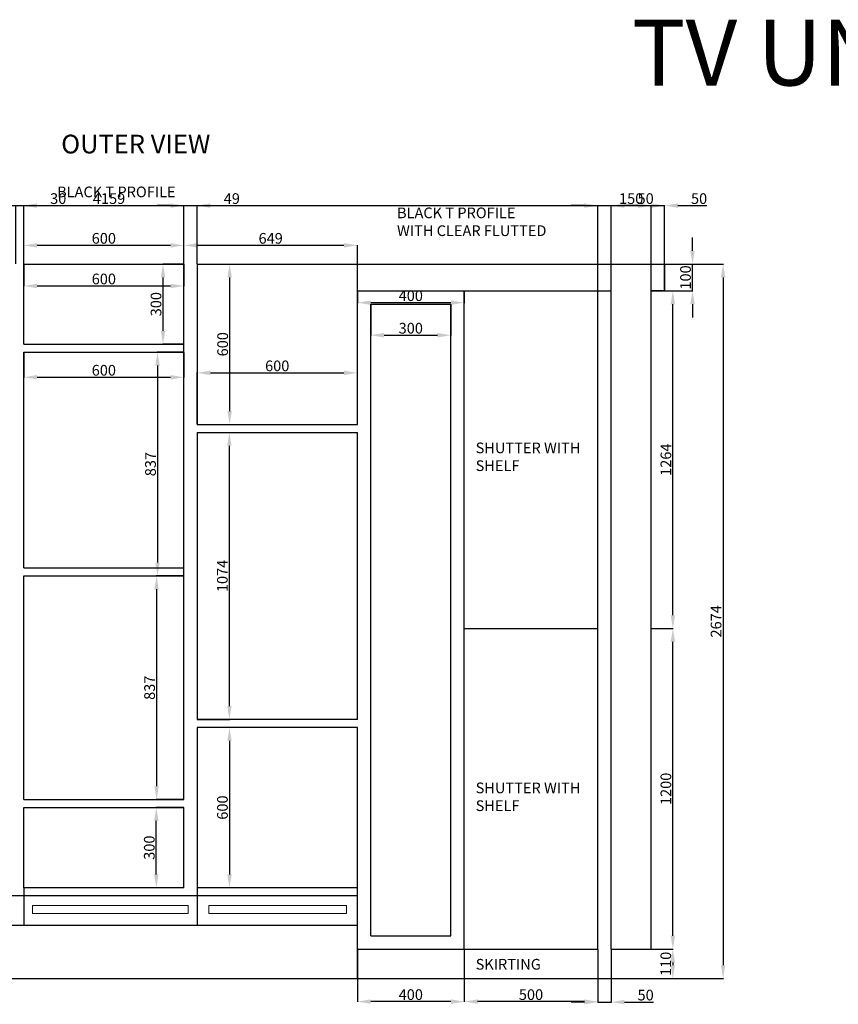
# Model space of a CAD drawing. Units: millimetres. Extents: x -2182 to 7969, y 257 to 4097.
# Tile 2 of 5: x -171 to 2894, y 412 to 4097. Entities that reach past the tile are written whole.
import ezdxf

# ---------------------------------------------------------------- set-up
doc = ezdxf.new("R2010")
doc.units = ezdxf.units.MM
for name, color, linetype, lineweight in [('A-ANNO-DIMS', 2, 'Continuous', 18), ('A-ANNO-TEXT', 3, 'Continuous', 18), ('A-ELEV', 7, 'Continuous', 25), ('A-FURN-HRDW', 8, 'Continuous', 18)]:
    doc.layers.add(name, color=color, linetype=linetype, lineweight=lineweight)
doc.styles.get("Standard").update_dxf_attribs({"font": 'arial.ttf'})
doc.dimstyles.new('ISO-25', dxfattribs={"dimtxt": 40, "dimasz": 50, "dimexe": 1.25, "dimexo": 0.625, "dimtad": 1, "dimtxsty": 'Standard', "dimcen": 2.5, "dimadec": 0, "dimazin": 0, "dimtfac": 1, "dimtmove": 0, "dimatfit": 3, "dimfxl": 1, "dimarcsym": 0})

# ---------------------------------------------------------------- blocks, each defined once
blk = doc.blocks.new('*D5')
at = {"layer": 'A-ANNO-DIMS', "color": 0, "lineweight": -2, "transparency": 16777216}
for p, q in [((2193.8, 618.5), (2275.3, 618.5)), ((2274.1, 568.5), (2274.1, 558.5)), ((2193.8, 508.5), (2275.3, 508.5))]:
    blk.add_line(p, q, dxfattribs=at)
at = {"layer": 'A-ANNO-DIMS', "color": 0, "transparency": 16777216}
for points in [[(2265.7, 568.5), (2282.4, 568.5), (2274.1, 618.5)], [(2265.7, 558.5), (2282.4, 558.5), (2274.1, 508.5)]]:
    blk.add_solid(points, dxfattribs=at)
at = {"layer": 'Defpoints', "color": 0, "transparency": 16777216}
for p in [(2193.2, 618.5), (2193.2, 508.5), (2274.1, 508.5)]:
    blk.add_point(p, dxfattribs=at)
at = {"layer": 'A-ANNO-DIMS', "color": 0, "transparency": 16777216, "insert": (2253, 563.5), "char_height": 40, "attachment_point": 5, "rotation": 90}
blk.add_mtext('110', dxfattribs=at)
blk = doc.blocks.new('*D6')
at = {"layer": 'A-ANNO-DIMS', "color": 0, "lineweight": -2, "transparency": 16777216}
for p, q in [((2193.8, 1818.5), (2275.6, 1818.5)), ((2274.3, 668.5), (2274.3, 1768.5)), ((2043.8, 618.5), (2275.6, 618.5))]:
    blk.add_line(p, q, dxfattribs=at)
at = {"layer": 'A-ANNO-DIMS', "color": 0, "transparency": 16777216}
for points in [[(2266, 1768.5), (2282.6, 1768.5), (2274.3, 1818.5)], [(2266, 668.5), (2282.6, 668.5), (2274.3, 618.5)]]:
    blk.add_solid(points, dxfattribs=at)
at = {"layer": 'Defpoints', "color": 0, "transparency": 16777216}
for p in [(2193.2, 1818.5), (2274.3, 1818.5), (2043.2, 618.5)]:
    blk.add_point(p, dxfattribs=at)
at = {"layer": 'A-ANNO-DIMS', "color": 0, "transparency": 16777216, "insert": (2253.3, 1218.5), "char_height": 40, "attachment_point": 5, "rotation": 90}
blk.add_mtext('1200', dxfattribs=at)
blk = doc.blocks.new('*D7')
at = {"layer": 'A-ANNO-DIMS', "color": 0, "lineweight": -2, "transparency": 16777216}
for p, q in [((2193.8, 3082.5), (2275.6, 3082.5)), ((2274.3, 1868.5), (2274.3, 3032.5)), ((2193.8, 1818.5), (2275.6, 1818.5))]:
    blk.add_line(p, q, dxfattribs=at)
at = {"layer": 'A-ANNO-DIMS', "color": 0, "transparency": 16777216}
for points in [[(2266, 3032.5), (2282.6, 3032.5), (2274.3, 3082.5)], [(2266, 1868.5), (2282.6, 1868.5), (2274.3, 1818.5)]]:
    blk.add_solid(points, dxfattribs=at)
at = {"layer": 'Defpoints', "color": 0, "transparency": 16777216}
for p in [(2193.2, 3082.5), (2274.3, 3082.5), (2193.2, 1818.5)]:
    blk.add_point(p, dxfattribs=at)
at = {"layer": 'A-ANNO-DIMS', "color": 0, "transparency": 16777216, "insert": (2253.3, 2450.5), "char_height": 40, "attachment_point": 5, "rotation": 90}
blk.add_mtext('1264', dxfattribs=at)
blk = doc.blocks.new('*D8')
at = {"layer": 'A-ANNO-DIMS', "color": 0, "lineweight": -2, "transparency": 16777216}
for p, q in [((2347.9, 3232.5), (2347.9, 3282.5)), ((2243.8, 3182.5), (2349.1, 3182.5)), ((2347.9, 3082.5), (2347.9, 3182.5)), ((2245.1, 3082.5), (2349.1, 3082.5)), ((2347.9, 3032.5), (2347.9, 2982.5))]:
    blk.add_line(p, q, dxfattribs=at)
at = {"layer": 'A-ANNO-DIMS', "color": 0, "transparency": 16777216}
for points in [[(2339.6, 3232.5), (2356.2, 3232.5), (2347.9, 3182.5)], [(2339.6, 3032.5), (2356.2, 3032.5), (2347.9, 3082.5)]]:
    blk.add_solid(points, dxfattribs=at)
at = {"layer": 'Defpoints', "color": 0, "transparency": 16777216}
for p in [(2243.2, 3182.5), (2347.9, 3182.5), (2244.4, 3082.5)]:
    blk.add_point(p, dxfattribs=at)
at = {"layer": 'A-ANNO-DIMS', "color": 0, "transparency": 16777216, "insert": (2326.8, 3132.5), "char_height": 40, "attachment_point": 5, "rotation": 90}
blk.add_mtext('100', dxfattribs=at)
blk = doc.blocks.new('*D9')
at = {"layer": 'A-ANNO-DIMS', "color": 0, "lineweight": -2, "transparency": 16777216}
for p, q in [((1993.2, 617.8), (1993.2, 419.3)), ((2043.2, 617.8), (2043.2, 419.3)), ((1943.2, 420.5), (1893.2, 420.5)), ((1993.2, 420.5), (2043.2, 420.5)), ((2093.2, 420.5), (2201.6, 420.5))]:
    blk.add_line(p, q, dxfattribs=at)
at = {"layer": 'A-ANNO-DIMS', "color": 0, "transparency": 16777216}
for points in [[(1943.2, 428.9), (1943.2, 412.2), (1993.2, 420.5)], [(2093.2, 428.9), (2093.2, 412.2), (2043.2, 420.5)]]:
    blk.add_solid(points, dxfattribs=at)
at = {"layer": 'Defpoints', "color": 0, "transparency": 16777216}
for p in [(1993.2, 618.5), (2043.2, 618.5), (1993.2, 420.5)]:
    blk.add_point(p, dxfattribs=at)
at = {"layer": 'A-ANNO-DIMS', "color": 0, "transparency": 16777216, "insert": (2172.4, 441.6), "char_height": 40, "attachment_point": 5}
blk.add_mtext('50', dxfattribs=at)
blk = doc.blocks.new('*D10')
at = {"layer": 'A-ANNO-DIMS', "color": 0, "lineweight": -2, "transparency": 16777216}
for p, q in [((1493.2, 617.8), (1493.2, 421)), ((1993.2, 617.8), (1993.2, 421)), ((1943.2, 422.3), (1543.2, 422.3))]:
    blk.add_line(p, q, dxfattribs=at)
at = {"layer": 'A-ANNO-DIMS', "color": 0, "transparency": 16777216}
for points in [[(1543.2, 430.6), (1543.2, 413.9), (1493.2, 422.3)], [(1943.2, 430.6), (1943.2, 413.9), (1993.2, 422.3)]]:
    blk.add_solid(points, dxfattribs=at)
at = {"layer": 'Defpoints', "color": 0, "transparency": 16777216}
for p in [(1493.2, 618.5), (1993.2, 618.5), (1493.2, 422.3)]:
    blk.add_point(p, dxfattribs=at)
at = {"layer": 'A-ANNO-DIMS', "color": 0, "transparency": 16777216, "insert": (1743.2, 443.3), "char_height": 40, "attachment_point": 5}
blk.add_mtext('500', dxfattribs=at)
blk = doc.blocks.new('*D11')
at = {"layer": 'A-ANNO-DIMS', "color": 0, "lineweight": -2, "transparency": 16777216}
for p, q in [((1093.2, 617.8), (1093.2, 421)), ((1493.2, 617.8), (1493.2, 421)), ((1443.2, 422.3), (1143.2, 422.3))]:
    blk.add_line(p, q, dxfattribs=at)
at = {"layer": 'A-ANNO-DIMS', "color": 0, "transparency": 16777216}
for points in [[(1143.2, 430.6), (1143.2, 413.9), (1093.2, 422.3)], [(1443.2, 430.6), (1443.2, 413.9), (1493.2, 422.3)]]:
    blk.add_solid(points, dxfattribs=at)
at = {"layer": 'Defpoints', "color": 0, "transparency": 16777216}
for p in [(1093.2, 618.5), (1493.2, 618.5), (1093.2, 422.3)]:
    blk.add_point(p, dxfattribs=at)
at = {"layer": 'A-ANNO-DIMS', "color": 0, "transparency": 16777216, "insert": (1293.2, 443.3), "char_height": 40, "attachment_point": 5}
blk.add_mtext('400', dxfattribs=at)
blk = doc.blocks.new('*D12')
at = {"layer": 'A-ANNO-DIMS', "color": 0, "lineweight": -2, "transparency": 16777216}
for p, q in [((493.2, 2583.1), (493.2, 2776.7)), ((543.2, 2775.4), (1043.2, 2775.4)), ((1093.2, 2583.1), (1093.2, 2776.7))]:
    blk.add_line(p, q, dxfattribs=at)
at = {"layer": 'A-ANNO-DIMS', "color": 0, "transparency": 16777216}
for points in [[(543.2, 2783.8), (543.2, 2767.1), (493.2, 2775.4)], [(1043.2, 2783.8), (1043.2, 2767.1), (1093.2, 2775.4)]]:
    blk.add_solid(points, dxfattribs=at)
at = {"layer": 'Defpoints', "color": 0, "transparency": 16777216}
for p in [(1093.2, 2775.4), (493.2, 2582.5), (1093.2, 2582.5)]:
    blk.add_point(p, dxfattribs=at)
at = {"layer": 'A-ANNO-DIMS', "color": 0, "transparency": 16777216, "insert": (793.2, 2796.5), "char_height": 40, "attachment_point": 5}
blk.add_mtext('600', dxfattribs=at)
blk = doc.blocks.new('*D13')
at = {"layer": 'A-ANNO-DIMS', "color": 0, "lineweight": -2, "transparency": 16777216}
for p, q in [((493.8, 3182.5), (616.4, 3182.5)), ((615.1, 3132.5), (615.1, 2632.5)), ((493.8, 2582.5), (616.4, 2582.5))]:
    blk.add_line(p, q, dxfattribs=at)
at = {"layer": 'A-ANNO-DIMS', "color": 0, "transparency": 16777216}
for points in [[(606.8, 3132.5), (623.5, 3132.5), (615.1, 3182.5)], [(606.8, 2632.5), (623.5, 2632.5), (615.1, 2582.5)]]:
    blk.add_solid(points, dxfattribs=at)
at = {"layer": 'Defpoints', "color": 0, "transparency": 16777216}
for p in [(493.2, 3182.5), (493.2, 2582.5), (615.1, 2582.5)]:
    blk.add_point(p, dxfattribs=at)
at = {"layer": 'A-ANNO-DIMS', "color": 0, "transparency": 16777216, "insert": (594.1, 2882.5), "char_height": 40, "attachment_point": 5, "rotation": 90}
blk.add_mtext('600', dxfattribs=at)
blk = doc.blocks.new('*D14')
at = {"layer": 'A-ANNO-DIMS', "color": 0, "lineweight": -2, "transparency": 16777216}
for p, q in [((493.8, 2552.5), (615.3, 2552.5)), ((614.1, 1528.5), (614.1, 2502.5)), ((493.8, 1478.5), (615.3, 1478.5))]:
    blk.add_line(p, q, dxfattribs=at)
at = {"layer": 'A-ANNO-DIMS', "color": 0, "transparency": 16777216}
for points in [[(605.8, 2502.5), (622.4, 2502.5), (614.1, 2552.5)], [(605.8, 1528.5), (622.4, 1528.5), (614.1, 1478.5)]]:
    blk.add_solid(points, dxfattribs=at)
at = {"layer": 'Defpoints', "color": 0, "transparency": 16777216}
for p in [(493.2, 2552.5), (614.1, 2552.5), (493.2, 1478.5)]:
    blk.add_point(p, dxfattribs=at)
at = {"layer": 'A-ANNO-DIMS', "color": 0, "transparency": 16777216, "insert": (593, 2015.5), "char_height": 40, "attachment_point": 5, "rotation": 90}
blk.add_mtext('1074', dxfattribs=at)
blk = doc.blocks.new('*D15')
at = {"layer": 'A-ANNO-DIMS', "color": 0, "lineweight": -2, "transparency": 16777216}
for p, q in [((792.6, 1448.5), (613.2, 1448.5)), ((614.5, 1398.5), (614.5, 898.5)), ((792.6, 848.5), (613.2, 848.5))]:
    blk.add_line(p, q, dxfattribs=at)
at = {"layer": 'A-ANNO-DIMS', "color": 0, "transparency": 16777216}
for points in [[(606.2, 1398.5), (622.8, 1398.5), (614.5, 1448.5)], [(606.2, 898.5), (622.8, 898.5), (614.5, 848.5)]]:
    blk.add_solid(points, dxfattribs=at)
at = {"layer": 'Defpoints', "color": 0, "transparency": 16777216}
for p in [(793.2, 1448.5), (614.5, 848.5), (793.2, 848.5)]:
    blk.add_point(p, dxfattribs=at)
at = {"layer": 'A-ANNO-DIMS', "color": 0, "transparency": 16777216, "insert": (593.4, 1148.5), "char_height": 40, "attachment_point": 5, "rotation": 90}
blk.add_mtext('600', dxfattribs=at)
blk = doc.blocks.new('*D16')
at = {"layer": 'A-ANNO-DIMS', "color": 0, "lineweight": -2, "transparency": 16777216}
for p, q in [((444.2, 3183.1), (444.2, 3254)), ((1043.2, 3252.7), (494.2, 3252.7)), ((1093.2, 3183.1), (1093.2, 3254))]:
    blk.add_line(p, q, dxfattribs=at)
at = {"layer": 'A-ANNO-DIMS', "color": 0, "transparency": 16777216}
for points in [[(494.2, 3261.1), (494.2, 3244.4), (444.2, 3252.7)], [(1043.2, 3261.1), (1043.2, 3244.4), (1093.2, 3252.7)]]:
    blk.add_solid(points, dxfattribs=at)
at = {"layer": 'Defpoints', "color": 0, "transparency": 16777216}
for p in [(444.2, 3252.7), (444.2, 3182.5), (1093.2, 3182.5)]:
    blk.add_point(p, dxfattribs=at)
at = {"layer": 'A-ANNO-DIMS', "color": 0, "transparency": 16777216, "insert": (768.7, 3273.8), "char_height": 40, "attachment_point": 5}
blk.add_mtext('649', dxfattribs=at)
blk = doc.blocks.new('*D17')
at = {"layer": 'A-ANNO-DIMS', "color": 0, "lineweight": -2, "transparency": 16777216}
for p, q in [((443.6, 3182.5), (364.6, 3182.5)), ((365.8, 2932.5), (365.8, 3132.5)), ((443.6, 2882.5), (364.6, 2882.5))]:
    blk.add_line(p, q, dxfattribs=at)
at = {"layer": 'A-ANNO-DIMS', "color": 0, "transparency": 16777216}
for points in [[(357.5, 3132.5), (374.1, 3132.5), (365.8, 3182.5)], [(357.5, 2932.5), (374.1, 2932.5), (365.8, 2882.5)]]:
    blk.add_solid(points, dxfattribs=at)
at = {"layer": 'Defpoints', "color": 0, "transparency": 16777216}
for p in [(365.8, 3182.5), (444.2, 3182.5), (444.2, 2882.5)]:
    blk.add_point(p, dxfattribs=at)
at = {"layer": 'A-ANNO-DIMS', "color": 0, "transparency": 16777216, "insert": (344.7, 3032.5), "char_height": 40, "attachment_point": 5, "rotation": 90}
blk.add_mtext('300', dxfattribs=at)
blk = doc.blocks.new('*D18')
at = {"layer": 'A-ANNO-DIMS', "color": 0, "lineweight": -2, "transparency": 16777216}
for p, q in [((-155.8, 2851.8), (-155.8, 2757.7)), ((444.2, 2851.8), (444.2, 2757.7)), ((-105.8, 2759), (394.2, 2759))]:
    blk.add_line(p, q, dxfattribs=at)
at = {"layer": 'A-ANNO-DIMS', "color": 0, "transparency": 16777216}
for points in [[(-105.8, 2767.3), (-105.8, 2750.6), (-155.8, 2759)], [(394.2, 2767.3), (394.2, 2750.6), (444.2, 2759)]]:
    blk.add_solid(points, dxfattribs=at)
at = {"layer": 'Defpoints', "color": 0, "transparency": 16777216}
for p in [(-155.8, 2852.5), (444.2, 2852.5), (444.2, 2759)]:
    blk.add_point(p, dxfattribs=at)
at = {"layer": 'A-ANNO-DIMS', "color": 0, "transparency": 16777216, "insert": (144.2, 2780), "char_height": 40, "attachment_point": 5}
blk.add_mtext('600', dxfattribs=at)
blk = doc.blocks.new('*D19')
at = {"layer": 'A-ANNO-DIMS', "color": 0, "lineweight": -2, "transparency": 16777216}
for p, q in [((443.6, 2852.5), (343.9, 2852.5)), ((345.2, 2802.5), (345.2, 2065.5)), ((443.6, 2015.5), (343.9, 2015.5))]:
    blk.add_line(p, q, dxfattribs=at)
at = {"layer": 'A-ANNO-DIMS', "color": 0, "transparency": 16777216}
for points in [[(336.8, 2802.5), (353.5, 2802.5), (345.2, 2852.5)], [(336.8, 2065.5), (353.5, 2065.5), (345.2, 2015.5)]]:
    blk.add_solid(points, dxfattribs=at)
at = {"layer": 'Defpoints', "color": 0, "transparency": 16777216}
for p in [(444.2, 2852.5), (345.2, 2015.5), (444.2, 2015.5)]:
    blk.add_point(p, dxfattribs=at)
at = {"layer": 'A-ANNO-DIMS', "color": 0, "transparency": 16777216, "insert": (324.1, 2434), "char_height": 40, "attachment_point": 5, "rotation": 90}
blk.add_mtext('837', dxfattribs=at)
blk = doc.blocks.new('*D20')
at = {"layer": 'A-ANNO-DIMS', "color": 0, "lineweight": -2, "transparency": 16777216}
for p, q in [((-155.8, 3181.8), (-155.8, 3099.4)), ((444.2, 3181.8), (444.2, 3099.4)), ((-105.8, 3100.7), (394.2, 3100.7))]:
    blk.add_line(p, q, dxfattribs=at)
at = {"layer": 'A-ANNO-DIMS', "color": 0, "transparency": 16777216}
for points in [[(-105.8, 3109), (-105.8, 3092.3), (-155.8, 3100.7)], [(394.2, 3109), (394.2, 3092.3), (444.2, 3100.7)]]:
    blk.add_solid(points, dxfattribs=at)
at = {"layer": 'Defpoints', "color": 0, "transparency": 16777216}
for p in [(-155.8, 3182.5), (444.2, 3182.5), (444.2, 3100.7)]:
    blk.add_point(p, dxfattribs=at)
at = {"layer": 'A-ANNO-DIMS', "color": 0, "transparency": 16777216, "insert": (144.2, 3121.7), "char_height": 40, "attachment_point": 5}
blk.add_mtext('600', dxfattribs=at)
blk = doc.blocks.new('*D21')
at = {"layer": 'A-ANNO-DIMS', "color": 0, "lineweight": -2, "transparency": 16777216}
for p, q in [((443.6, 2015.5), (340.4, 2015.5)), ((341.6, 1965.5), (341.6, 1228.5)), ((443.6, 1178.5), (340.4, 1178.5))]:
    blk.add_line(p, q, dxfattribs=at)
at = {"layer": 'A-ANNO-DIMS', "color": 0, "transparency": 16777216}
for points in [[(333.3, 1965.5), (349.9, 1965.5), (341.6, 2015.5)], [(333.3, 1228.5), (349.9, 1228.5), (341.6, 1178.5)]]:
    blk.add_solid(points, dxfattribs=at)
at = {"layer": 'Defpoints', "color": 0, "transparency": 16777216}
for p in [(444.2, 2015.5), (341.6, 1178.5), (444.2, 1178.5)]:
    blk.add_point(p, dxfattribs=at)
at = {"layer": 'A-ANNO-DIMS', "color": 0, "transparency": 16777216, "insert": (320.6, 1597), "char_height": 40, "attachment_point": 5, "rotation": 90}
blk.add_mtext('837', dxfattribs=at)
blk = doc.blocks.new('*D22')
at = {"layer": 'A-ANNO-DIMS', "color": 0, "lineweight": -2, "transparency": 16777216}
for p, q in [((443.6, 1148.5), (339.3, 1148.5)), ((340.6, 898.5), (340.6, 1098.5)), ((443.6, 848.5), (339.3, 848.5))]:
    blk.add_line(p, q, dxfattribs=at)
at = {"layer": 'A-ANNO-DIMS', "color": 0, "transparency": 16777216}
for points in [[(332.2, 1098.5), (348.9, 1098.5), (340.6, 1148.5)], [(332.2, 898.5), (348.9, 898.5), (340.6, 848.5)]]:
    blk.add_solid(points, dxfattribs=at)
at = {"layer": 'Defpoints', "color": 0, "transparency": 16777216}
for p in [(340.6, 1148.5), (444.2, 1148.5), (444.2, 848.5)]:
    blk.add_point(p, dxfattribs=at)
at = {"layer": 'A-ANNO-DIMS', "color": 0, "transparency": 16777216, "insert": (319.5, 998.5), "char_height": 40, "attachment_point": 5, "rotation": 90}
blk.add_mtext('300', dxfattribs=at)
blk = doc.blocks.new('*D23')
at = {"layer": 'A-ANNO-DIMS', "color": 0, "lineweight": -2, "transparency": 16777216}
for p, q in [((-155.8, 3183.1), (-155.8, 3253.9)), ((394.2, 3252.6), (-105.8, 3252.6)), ((444.2, 3183.1), (444.2, 3253.9))]:
    blk.add_line(p, q, dxfattribs=at)
at = {"layer": 'A-ANNO-DIMS', "color": 0, "transparency": 16777216}
for points in [[(-105.8, 3261), (-105.8, 3244.3), (-155.8, 3252.6)], [(394.2, 3261), (394.2, 3244.3), (444.2, 3252.6)]]:
    blk.add_solid(points, dxfattribs=at)
at = {"layer": 'Defpoints', "color": 0, "transparency": 16777216}
for p in [(-155.8, 3252.6), (-155.8, 3182.5), (444.2, 3182.5)]:
    blk.add_point(p, dxfattribs=at)
at = {"layer": 'A-ANNO-DIMS', "color": 0, "transparency": 16777216, "insert": (144.2, 3273.7), "char_height": 40, "attachment_point": 5}
blk.add_mtext('600', dxfattribs=at)
blk = doc.blocks.new('*D55')
at = {"layer": 'A-ANNO-DIMS', "color": 0, "lineweight": -2, "transparency": 16777216}
for p, q in [((1143.2, 3031.8), (1143.2, 2915.1)), ((1443.2, 3031.8), (1443.2, 2915.1)), ((1193.2, 2916.3), (1393.2, 2916.3))]:
    blk.add_line(p, q, dxfattribs=at)
at = {"layer": 'A-ANNO-DIMS', "color": 0, "transparency": 16777216}
for points in [[(1193.2, 2924.6), (1193.2, 2908), (1143.2, 2916.3)], [(1393.2, 2924.6), (1393.2, 2908), (1443.2, 2916.3)]]:
    blk.add_solid(points, dxfattribs=at)
at = {"layer": 'Defpoints', "color": 0, "transparency": 16777216}
for p in [(1143.2, 3032.5), (1443.2, 3032.5), (1443.2, 2916.3)]:
    blk.add_point(p, dxfattribs=at)
at = {"layer": 'A-ANNO-DIMS', "color": 0, "transparency": 16777216, "insert": (1293.2, 2937.4), "char_height": 40, "attachment_point": 5}
blk.add_mtext('300', dxfattribs=at)
blk = doc.blocks.new('*D56')
at = {"layer": 'A-ANNO-DIMS', "color": 0, "lineweight": -2, "transparency": 16777216}
for p, q in [((1093.2, 3081.8), (1093.2, 3036.9)), ((1493.2, 3081.8), (1493.2, 3036.9)), ((1443.2, 3038.1), (1143.2, 3038.1))]:
    blk.add_line(p, q, dxfattribs=at)
at = {"layer": 'A-ANNO-DIMS', "color": 0, "transparency": 16777216}
for points in [[(1143.2, 3046.5), (1143.2, 3029.8), (1093.2, 3038.1)], [(1443.2, 3046.5), (1443.2, 3029.8), (1493.2, 3038.1)]]:
    blk.add_solid(points, dxfattribs=at)
at = {"layer": 'Defpoints', "color": 0, "transparency": 16777216}
for p in [(1093.2, 3082.5), (1493.2, 3082.5), (1093.2, 3038.1)]:
    blk.add_point(p, dxfattribs=at)
at = {"layer": 'A-ANNO-DIMS', "color": 0, "transparency": 16777216, "insert": (1293.2, 3059.2), "char_height": 40, "attachment_point": 5}
blk.add_mtext('400', dxfattribs=at)
blk = doc.blocks.new('*D64')
at = {"layer": 'A-ANNO-DIMS', "color": 0, "lineweight": -2, "transparency": 16777216}
for p, q in [((-1915.8, 509.1), (-1915.8, 3402.7)), ((-1865.8, 3401.5), (2193.2, 3401.5)), ((2243.2, 3183.1), (2243.2, 3402.7))]:
    blk.add_line(p, q, dxfattribs=at)
at = {"layer": 'A-ANNO-DIMS', "color": 0, "transparency": 16777216}
for points in [[(-1865.8, 3409.8), (-1865.8, 3393.1), (-1915.8, 3401.5)], [(2193.2, 3409.8), (2193.2, 3393.1), (2243.2, 3401.5)]]:
    blk.add_solid(points, dxfattribs=at)
at = {"layer": 'Defpoints', "color": 0, "transparency": 16777216}
for p in [(2243.2, 3401.5), (2243.2, 3182.5), (-1915.8, 508.5)]:
    blk.add_point(p, dxfattribs=at)
at = {"layer": 'A-ANNO-DIMS', "color": 0, "transparency": 16777216, "insert": (163.7, 3422.5), "char_height": 40, "attachment_point": 5}
blk.add_mtext('4159', dxfattribs=at)
blk = doc.blocks.new('*D65')
at = {"layer": 'A-ANNO-DIMS', "color": 0, "lineweight": -2, "transparency": 16777216}
for p, q in [((2243.8, 3182.5), (2463.4, 3182.5)), ((2462.2, 3132.5), (2462.2, 558.5)), ((2193.8, 508.5), (2463.4, 508.5))]:
    blk.add_line(p, q, dxfattribs=at)
at = {"layer": 'A-ANNO-DIMS', "color": 0, "transparency": 16777216}
for points in [[(2453.9, 3132.5), (2470.5, 3132.5), (2462.2, 3182.5)], [(2453.9, 558.5), (2470.5, 558.5), (2462.2, 508.5)]]:
    blk.add_solid(points, dxfattribs=at)
at = {"layer": 'Defpoints', "color": 0, "transparency": 16777216}
for p in [(2243.2, 3182.5), (2193.2, 508.5), (2462.2, 508.5)]:
    blk.add_point(p, dxfattribs=at)
at = {"layer": 'A-ANNO-DIMS', "color": 0, "transparency": 16777216, "insert": (2441.1, 1845.5), "char_height": 40, "attachment_point": 5, "rotation": 90}
blk.add_mtext('2674', dxfattribs=at)
blk = doc.blocks.new('*D69')
at = {"layer": 'A-ANNO-DIMS', "color": 0, "lineweight": -2, "transparency": 16777216}
for p, q in [((-235.8, 3401.5), (-285.8, 3401.5)), ((-185.8, 3183.1), (-185.8, 3402.7)), ((-185.8, 3401.5), (-155.8, 3401.5)), ((-155.8, 3183.1), (-155.8, 3402.7)), ((-105.8, 3401.5), (2.6, 3401.5))]:
    blk.add_line(p, q, dxfattribs=at)
at = {"layer": 'A-ANNO-DIMS', "color": 0, "transparency": 16777216}
for points in [[(-235.8, 3409.8), (-235.8, 3393.1), (-185.8, 3401.5)], [(-105.8, 3409.8), (-105.8, 3393.1), (-155.8, 3401.5)]]:
    blk.add_solid(points, dxfattribs=at)
at = {"layer": 'Defpoints', "color": 0, "transparency": 16777216}
for p in [(-155.8, 3401.5), (-185.8, 3182.5), (-155.8, 3182.5)]:
    blk.add_point(p, dxfattribs=at)
at = {"layer": 'A-ANNO-DIMS', "color": 0, "transparency": 16777216, "insert": (-26.6, 3422.5), "char_height": 40, "attachment_point": 5}
blk.add_mtext('30', dxfattribs=at)
blk = doc.blocks.new('*D70')
at = {"layer": 'A-ANNO-DIMS', "color": 0, "lineweight": -2, "transparency": 16777216}
for p, q in [((394.2, 3401.5), (344.2, 3401.5)), ((444.2, 3183.1), (444.2, 3402.7)), ((444.2, 3401.5), (493.2, 3401.5)), ((493.2, 3183.1), (493.2, 3402.7)), ((543.2, 3401.5), (653.4, 3401.5))]:
    blk.add_line(p, q, dxfattribs=at)
at = {"layer": 'A-ANNO-DIMS', "color": 0, "transparency": 16777216}
for points in [[(394.2, 3409.8), (394.2, 3393.1), (444.2, 3401.5)], [(543.2, 3409.8), (543.2, 3393.1), (493.2, 3401.5)]]:
    blk.add_solid(points, dxfattribs=at)
at = {"layer": 'Defpoints', "color": 0, "transparency": 16777216}
for p in [(493.2, 3401.5), (444.2, 3182.5), (493.2, 3182.5)]:
    blk.add_point(p, dxfattribs=at)
at = {"layer": 'A-ANNO-DIMS', "color": 0, "transparency": 16777216, "insert": (623.3, 3422.5), "char_height": 40, "attachment_point": 5}
blk.add_mtext('49', dxfattribs=at)
blk = doc.blocks.new('*D71')
at = {"layer": 'A-ANNO-DIMS', "color": 0, "lineweight": -2, "transparency": 16777216}
for p, q in [((1943.2, 3401.5), (1893.2, 3401.5)), ((1993.2, 3083.1), (1993.2, 3402.7)), ((1993.2, 3401.5), (2043.2, 3401.5)), ((2043.2, 3083.1), (2043.2, 3402.7)), ((2093.2, 3401.5), (2201.6, 3401.5))]:
    blk.add_line(p, q, dxfattribs=at)
at = {"layer": 'A-ANNO-DIMS', "color": 0, "transparency": 16777216}
for points in [[(1943.2, 3409.8), (1943.2, 3393.1), (1993.2, 3401.5)], [(2093.2, 3409.8), (2093.2, 3393.1), (2043.2, 3401.5)]]:
    blk.add_solid(points, dxfattribs=at)
at = {"layer": 'Defpoints', "color": 0, "transparency": 16777216}
for p in [(2043.2, 3401.5), (1993.2, 3082.5), (2043.2, 3082.5)]:
    blk.add_point(p, dxfattribs=at)
at = {"layer": 'A-ANNO-DIMS', "color": 0, "transparency": 16777216, "insert": (2172.4, 3422.5), "char_height": 40, "attachment_point": 5}
blk.add_mtext('50', dxfattribs=at)
blk = doc.blocks.new('*D72')
at = {"layer": 'A-ANNO-DIMS', "color": 0, "lineweight": -2, "transparency": 16777216}
for p, q in [((2043.2, 3083.1), (2043.2, 3402.7)), ((2093.2, 3401.5), (2143.2, 3401.5)), ((2193.2, 3083.1), (2193.2, 3402.7))]:
    blk.add_line(p, q, dxfattribs=at)
at = {"layer": 'A-ANNO-DIMS', "color": 0, "transparency": 16777216}
for points in [[(2093.2, 3409.8), (2093.2, 3393.1), (2043.2, 3401.5)], [(2143.2, 3409.8), (2143.2, 3393.1), (2193.2, 3401.5)]]:
    blk.add_solid(points, dxfattribs=at)
at = {"layer": 'Defpoints', "color": 0, "transparency": 16777216}
for p in [(2193.2, 3401.5), (2043.2, 3082.5), (2193.2, 3082.5)]:
    blk.add_point(p, dxfattribs=at)
at = {"layer": 'A-ANNO-DIMS', "color": 0, "transparency": 16777216, "insert": (2118.2, 3422.5), "char_height": 40, "attachment_point": 5}
blk.add_mtext('150', dxfattribs=at)
blk = doc.blocks.new('*D73')
at = {"layer": 'A-ANNO-DIMS', "color": 0, "lineweight": -2, "transparency": 16777216}
for p, q in [((2143.2, 3401.5), (2093.2, 3401.5)), ((2193.2, 3083.1), (2193.2, 3402.7)), ((2193.2, 3401.5), (2243.2, 3401.5)), ((2243.2, 3083.1), (2243.2, 3402.7)), ((2293.2, 3401.5), (2401.6, 3401.5))]:
    blk.add_line(p, q, dxfattribs=at)
at = {"layer": 'A-ANNO-DIMS', "color": 0, "transparency": 16777216}
for points in [[(2143.2, 3409.8), (2143.2, 3393.1), (2193.2, 3401.5)], [(2293.2, 3409.8), (2293.2, 3393.1), (2243.2, 3401.5)]]:
    blk.add_solid(points, dxfattribs=at)
at = {"layer": 'Defpoints', "color": 0, "transparency": 16777216}
for p in [(2243.2, 3401.5), (2193.2, 3082.5), (2243.2, 3082.5)]:
    blk.add_point(p, dxfattribs=at)
at = {"layer": 'A-ANNO-DIMS', "color": 0, "transparency": 16777216, "insert": (2372.4, 3422.5), "char_height": 40, "attachment_point": 5}
blk.add_mtext('50', dxfattribs=at)

msp = doc.modelspace()

# ---------------------------------------------------------------- linework, layer by layer
at = {"layer": 'A-ELEV'}
for p, q in [((-155.8106, 3182.4543), (444.1894, 3182.4543)), ((-155.8106, 2882.4543), (-155.8106, 3182.4543)), ((444.1894, 1178.4543), (444.1894, 3182.4543)), ((493.1894, 3182.4543), (493.1894, 2582.4543)), ((493.1894, 3182.4543), (2243.1894, 3182.4543)), ((1093.1894, 2582.4543), (1093.1894, 3182.4543)), ((2243.1894, 3182.4543), (2243.1894, 3082.4543)), ((1093.1894, 3082.4543), (2043.1894, 3082.4543)), ((1493.1894, 618.4543), (1493.1894, 3082.4543)), ((1993.1894, 618.4543), (1993.1894, 3082.4543)), ((2043.1894, 618.4543), (2043.1894, 3082.4543)), ((2193.1894, 618.4543), (2193.1894, 3082.4543)), ((2243.1894, 3082.4543), (2193.1894, 3082.4543)), ((1143.1894, 668.4543), (1143.1894, 3032.4543)), ((1143.1894, 3032.4543), (1443.1894, 3032.4543)), ((1443.1894, 668.4543), (1443.1894, 3032.4543)), ((-155.8106, 2882.4543), (444.1894, 2882.4543)), ((-155.8106, 2852.4543), (444.1894, 2852.4543)), ((-155.8106, 2045.4543), (-155.8106, 2852.4543)), ((493.1894, 2582.4543), (1093.1894, 2582.4543)), ((493.1894, 2552.4543), (1093.1894, 2552.4543)), ((493.1894, 2552.4543), (493.1894, 1478.4543)), ((1093.1894, 1478.4543), (1093.1894, 2552.4543)), ((-155.8106, 2045.4543), (444.1894, 2045.4543)), ((-155.8106, 2015.4543), (444.1894, 2015.4543)), ((-155.8106, 1178.4543), (-155.8106, 2015.4543)), ((1493.1894, 1818.4543), (1993.1894, 1818.4543)), ((1093.1894, 1478.4543), (493.1894, 1478.4543)), ((1093.1894, 1448.4543), (493.1894, 1448.4543)), ((493.1894, 1448.4543), (493.1894, 848.4543)), ((1093.1894, 508.4543), (1093.1894, 1448.4543)), ((-155.8106, 1178.4543), (444.1894, 1178.4543)), ((-155.8106, 848.4543), (-155.8106, 1148.4543)), ((-155.8106, 1148.4543), (444.1894, 1148.4543)), ((444.1894, 848.4543), (444.1894, 1148.4543)), ((444.1894, 848.4543), (-155.8106, 848.4543)), ((-155.8106, 848.4543), (-155.8106, 708.4543)), ((1093.1894, 848.4543), (493.1894, 848.4543)), ((493.1894, 848.4543), (493.1894, 708.4543)), ((1093.1894, 818.4543), (-1415.8106, 818.4543)), ((-1915.8106, 708.4543), (1093.1894, 708.4543)), ((1143.1894, 668.4543), (1443.1894, 668.4543)), ((1093.1894, 618.4543), (1993.1894, 618.4543)), ((2043.1894, 618.4543), (2193.1894, 618.4543)), ((-1915.8106, 508.4543), (2193.1894, 508.4543))]:
    msp.add_line(p, q, dxfattribs=at)
at = {"layer": 'A-FURN-HRDW'}
for points in [[(-123.1886, 781.6689), (460.2077, 781.6689), (460.2077, 752.4682), (-123.1886, 752.4682)], [(537.0711, 781.6689), (1053.0207, 781.6689), (1053.0207, 752.4682), (537.0711, 752.4682)]]:
    msp.add_lwpolyline(points, close=True, dxfattribs=at)

# ---------------------------------------------------------------- texts
at = {"layer": 'A-ANNO-TEXT', "attachment_point": 1}
for s, insert, char_height, width in [('TV UNIT ', (2120.501, 4097.2574), 246.35353, 3842.081942), ('OUTER VIEW', (-15.4136, 3666.7691), 70, 1091.706432), ('BLACK T PROFILE', (-30.7647, 3472.658), 40, 482.986246), ('BLACK T PROFILE \\PWITH CLEAR FLUTTED ', (1241.6651, 3394.2304), 40, 716.323819), ('SHUTTER WITH \\PSHELF', (1535.9484, 2514.7205), 40, 482.986246), ('SHUTTER WITH \\PSHELF', (1535.9484, 1242.1887), 40, 482.986246), ('SKIRTING', (1535.9484, 582.0079), 40, 482.986246)]:
    msp.add_mtext(s, dxfattribs=dict(at, insert=insert, char_height=char_height, width=width))

# ---------------------------------------------------------------- dimensions: what is measured, and where the dimension line sits
at = {"layer": 'A-ANNO-DIMS'}
for base, p1, p2, override, picture, middle in [((2243.1894, 3401.4543), (-1915.8106, 508.4543), (2243.1894, 3182.4543), {"dimdec": 0, "dimlfac": 1, "dimrnd": 0, "dimzin": 0, "dimdsep": 46, "dimlunit": 2}, '*D64', (163.6894, 3422.5022)), ((-155.8106, 3401.4543), (-185.8106, 3182.4543), (-155.8106, 3182.4543), {"dimdec": 0, "dimlfac": 1, "dimrnd": 0, "dimzin": 0, "dimdsep": 46, "dimlunit": 2}, '*D69', (-26.6181, 3422.5159)), ((493.1894, 3401.4543), (444.1894, 3182.4543), (493.1894, 3182.4543), {"dimdec": 0, "dimlfac": 1, "dimrnd": 0, "dimzin": 0, "dimdsep": 46, "dimlunit": 2}, '*D70', (623.3096, 3422.5022)), ((2043.1894, 3401.4543), (1993.1894, 3082.4543), (2043.1894, 3082.4543), {"dimdec": 0, "dimlfac": 1, "dimrnd": 0, "dimzin": 0, "dimdsep": 46, "dimlunit": 2}, '*D71', (2172.3956, 3422.5022)), ((2193.1894, 3401.4543), (2043.1894, 3082.4543), (2193.1894, 3082.4543), {"dimdec": 0, "dimlfac": 1, "dimrnd": 0, "dimzin": 0, "dimdsep": 46, "dimlunit": 2}, '*D72', (2118.1894, 3422.5022)), ((2243.1894, 3401.4543), (2193.1894, 3082.4543), (2243.1894, 3082.4543), {"dimdec": 0, "dimlfac": 1, "dimrnd": 0, "dimzin": 0, "dimdsep": 46, "dimlunit": 2}, '*D73', (2372.3956, 3422.5022)), ((-155.8106, 3252.6206), (444.1894, 3182.4543), (-155.8106, 3182.4543), {"dimclrd": 0, "dimclre": 0, "dimclrt": 0}, '*D23', (144.1894, 3273.6685)), ((444.1894, 3252.736), (1093.1894, 3182.4543), (444.1894, 3182.4543), {"dimclrd": 0, "dimclre": 0, "dimclrt": 0}, '*D16', (768.6894, 3273.784)), ((444.1894, 3100.6599), (-155.8106, 3182.4543), (444.1894, 3182.4543), {"dimclrd": 0, "dimclre": 0, "dimclrt": 0}, '*D20', (144.1894, 3121.7078)), ((1093.1894, 3038.1236), (1493.1894, 3082.4543), (1093.1894, 3082.4543), {"dimclrd": 0, "dimclre": 0, "dimclrt": 0}, '*D56', (1293.1894, 3059.1715)), ((1443.1894, 2916.3099), (1143.1894, 3032.4543), (1443.1894, 3032.4543), {"dimclrd": 0, "dimclre": 0, "dimclrt": 0}, '*D55', (1293.1894, 2937.3715)), ((444.1894, 2758.9796), (-155.8106, 2852.4543), (444.1894, 2852.4543), {"dimclrd": 0, "dimclre": 0, "dimclrt": 0}, '*D18', (144.1894, 2780.0275)), ((1093.1894, 2775.4283), (493.1894, 2582.4543), (1093.1894, 2582.4543), {"dimclrd": 0, "dimclre": 0, "dimclrt": 0}, '*D12', (793.1894, 2796.4762)), ((1093.1894, 422.2734), (1493.1894, 618.4543), (1093.1894, 618.4543), {"dimclrd": 0, "dimclre": 0, "dimclrt": 0}, '*D11', (1293.1894, 443.3213)), ((1493.1894, 422.2734), (1993.1894, 618.4543), (1493.1894, 618.4543), {"dimclrd": 0, "dimclre": 0, "dimclrt": 0}, '*D10', (1743.1894, 443.3213))]:
    dim = msp.add_linear_dim(base=base, p1=p1, p2=p2, dimstyle='ISO-25', override=override, dxfattribs=at)
    dim.commit()
    dim.dimension.update_dxf_attribs({"geometry": picture, "text_midpoint": middle})
for base, p1, p2, picture, middle in [((2347.8932, 3182.4543), (2244.4394, 3082.4543), (2243.1894, 3182.4543), '*D8', (2347.8932, 3132.4543)), ((2274.0708, 508.4543), (2193.1894, 618.4543), (2193.1894, 508.4543), '*D5', (2274.0708, 563.4543))]:
    dim = msp.add_linear_dim(base=base, p1=p1, p2=p2, angle=90, dimstyle='ISO-25', override={"dimclrd": 0, "dimclre": 0, "dimclrt": 0}, dxfattribs=at)
    dim.commit()
    dim.dimension.update_dxf_attribs({"geometry": picture, "text_midpoint": middle, "dimtype": 160})
for base, p1, p2, override, picture, middle in [((365.8057, 3182.4543), (444.1894, 2882.4543), (444.1894, 3182.4543), {"dimclrd": 0, "dimclre": 0, "dimclrt": 0}, '*D17', (344.7441, 3032.4543)), ((615.121, 2582.4543), (493.1894, 3182.4543), (493.1894, 2582.4543), {"dimclrd": 0, "dimclre": 0, "dimclrt": 0}, '*D13', (594.0731, 2882.4543)), ((2462.1894, 508.4543), (2243.1894, 3182.4543), (2193.1894, 508.4543), {"dimdec": 0, "dimlfac": 1, "dimrnd": 0, "dimzin": 0, "dimdsep": 46, "dimlunit": 2}, '*D65', (2441.1415, 1845.4543)), ((2274.3164, 3082.4543), (2193.1894, 1818.4543), (2193.1894, 3082.4543), {"dimasz": 50, "dimclrd": 0, "dimclre": 0, "dimclrt": 0}, '*D7', (2253.2685, 2450.4543)), ((345.1711, 2015.4543), (444.1894, 2852.4543), (444.1894, 2015.4543), {"dimclrd": 0, "dimclre": 0, "dimclrt": 0}, '*D19', (324.1095, 2433.9543)), ((614.0976, 2552.4543), (493.1894, 1478.4543), (493.1894, 2552.4543), {"dimclrd": 0, "dimclre": 0, "dimclrt": 0}, '*D14', (593.0497, 2015.4543)), ((341.6166, 1178.4543), (444.1894, 2015.4543), (444.1894, 1178.4543), {"dimclrd": 0, "dimclre": 0, "dimclrt": 0}, '*D21', (320.5551, 1596.9543)), ((2274.3164, 1818.4543), (2043.1894, 618.4543), (2193.1894, 1818.4543), {"dimclrd": 0, "dimclre": 0, "dimclrt": 0}, '*D6', (2253.2685, 1218.4543)), ((614.4891, 848.4543), (793.1894, 1448.4543), (793.1894, 848.4543), {"dimclrd": 0, "dimclre": 0, "dimclrt": 0}, '*D15', (593.4412, 1148.4543)), ((340.5692, 1148.4543), (444.1894, 848.4543), (444.1894, 1148.4543), {"dimclrd": 0, "dimclre": 0, "dimclrt": 0}, '*D22', (319.5076, 998.4543))]:
    dim = msp.add_linear_dim(base=base, p1=p1, p2=p2, angle=90, dimstyle='ISO-25', override=override, dxfattribs=at)
    dim.commit()
    dim.dimension.update_dxf_attribs({"geometry": picture, "text_midpoint": middle})
dim = msp.add_linear_dim(base=(1993.1894, 420.5215), p1=(2043.1894, 618.4543), p2=(1993.1894, 618.4543), dimstyle='ISO-25', override={"dimclrd": 0, "dimclre": 0, "dimclrt": 0}, dxfattribs=at)
dim.commit()
dim.dimension.update_dxf_attribs({"geometry": '*D9', "text_midpoint": (2172.3956, 420.5215), "dimtype": 160})

doc.saveas('drawing.dxf')
